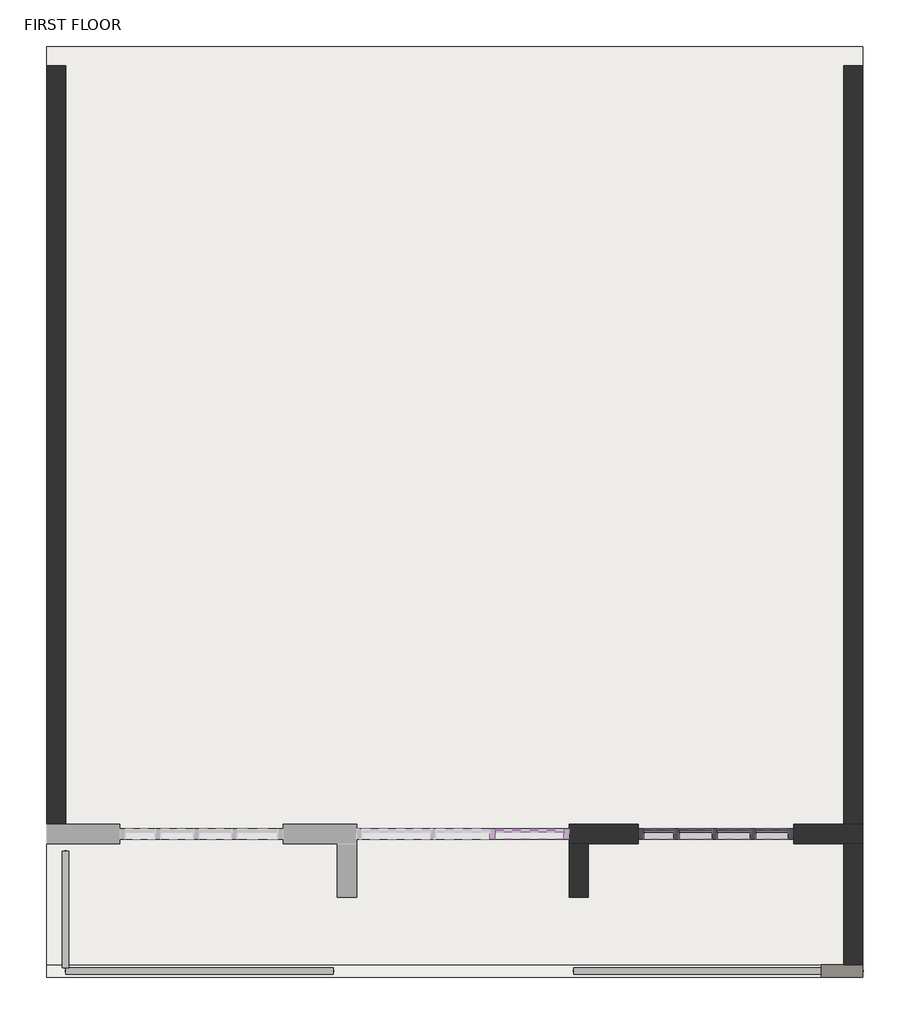
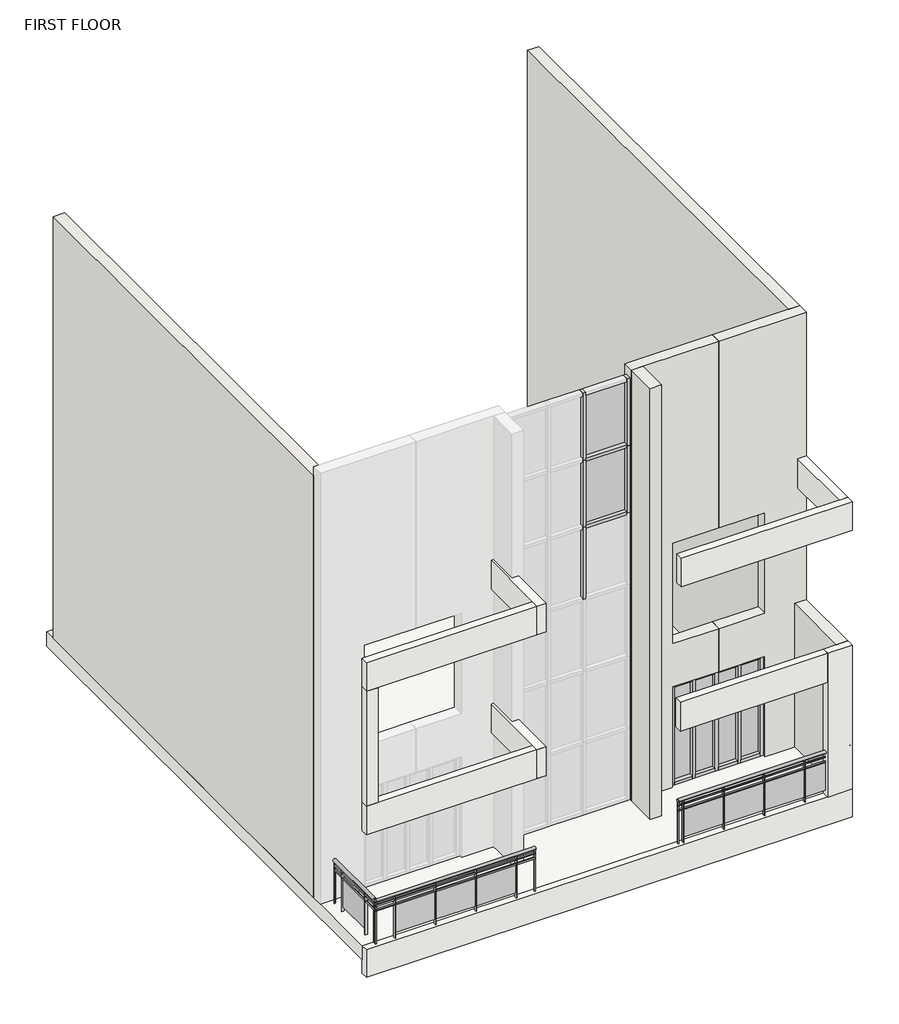
# One storey, part 2 of 2: 33 members, 10 plates, 6 walls, 3 railings, 2 slabs.
"""IFC4 building model written with IfcOpenShell, lengths in millimetres."""

from ifc_helpers import new_model, si_unit, point, frame, origin, place, context, project, spatial, polyline, ellipse_curve, trimmed, outline, extrude, faceted_brep, transform, mapped, element, save
from ifc_brep_helpers import plane_surface, extruded_surface, advanced_brep
from components import member_3374d9b6, member_ad567e07, member_82905deb, member_0514ece2, member_5493b72c, member_7cbddb58, member_843225dc, member_7096a90e, member_75a0f14a, system_panel_glazed_3f785c8f, system_panel_glazed_d91b2d6b, system_panel_glazed_935821d8, system_panel_glazed_f3f5655f, system_panel_glazed_451412b5, floors_1_floors_1_452276dc

model = new_model("IFC4")

# Units and contexts
model_context = context("Model", 3, world=origin())
ifc_project = project(units=[si_unit("LENGTHUNIT", "METRE", prefix="MILLI")], contexts=[model_context])

# Site, building, storey
site = spatial("IfcSite", under=ifc_project)
building = spatial("IfcBuilding", under=site)
storey = spatial("IfcBuildingStorey", under=building, Name="FIRST FLOOR", Elevation=3048.0)

# Members
placement = place(None, origin())
member_shape = member_3374d9b6(model_context)
element("IfcMember", 1, ObjectType="Rectangular Mullion : 2.5\" x 5\" rectangular", at=placement, inside=storey, context=model_context, shape_type="MappedRepresentation", body=[
    mapped(member_shape, transform((2606.0769214, -508.3464931, 3048.0), x_axis=(1.0, 0.0, 0.0), y_axis=(0.0, -1.0, 0.0), z_axis=(0.0, 0.0, -1.0))),
])
element("IfcMember", 2, ObjectType="Rectangular Mullion : 2.5\" x 5\" rectangular", at=placement, inside=storey, context=model_context, shape_type="MappedRepresentation", body=[
    mapped(member_shape, transform((2606.0769214, -508.3464931, 3048.0), x_axis=(1.0, 0.0, 0.0), y_axis=(0.0, -1.0, 0.0), z_axis=(0.0, 0.0, -1.0))),
])
element("IfcMember", 3, ObjectType="Rectangular Mullion : 2.5\" x 5\" rectangular", at=placement, inside=storey, context=model_context, shape_type="MappedRepresentation", body=[
    mapped(member_shape, transform((748.741197, -508.3464931, 5181.6), x_axis=(-1.0, 0.0, 0.0), y_axis=(0.0, -1.0, 0.0), z_axis=(0.0, 0.0, 1.0))),
])
element("IfcMember", 4, ObjectType="Rectangular Mullion : 2.5\" x 5\" rectangular", at=placement, inside=storey, context=model_context, shape_type="MappedRepresentation", body=[
    mapped(member_shape, transform((748.741197, -508.3464931, 5181.6), x_axis=(-1.0, 0.0, 0.0), y_axis=(0.0, -1.0, 0.0), z_axis=(0.0, 0.0, 1.0))),
])
member_2_shape = member_ad567e07(model_context)
element("IfcMember", 5, ObjectType="Rectangular Mullion : 2.5\" x 5\" rectangular", at=placement, inside=storey, context=model_context, shape_type="MappedRepresentation", body=[
    mapped(member_2_shape, transform((-140.258803, -508.3464931, 9144.0), x_axis=(0.0, 0.0, 1.0), y_axis=(0.0, -1.0, 0.0), z_axis=(1.0, 0.0, 0.0))),
])
element("IfcMember", 6, ObjectType="Rectangular Mullion : 2.5\" x 5\" rectangular", at=placement, inside=storey, context=model_context, shape_type="MappedRepresentation", body=[
    mapped(member_2_shape, transform((-140.258803, -508.3464931, 10572.1991558), x_axis=(0.0, 0.0, 1.0), y_axis=(0.0, -1.0, 0.0), z_axis=(1.0, 0.0, 0.0))),
])
member_3_shape = member_82905deb(model_context)
element("IfcMember", 7, ObjectType="Rectangular Mullion : 2.5\" x 5\" rectangular", at=placement, inside=storey, context=model_context, shape_type="MappedRepresentation", body=[
    mapped(member_3_shape, transform((-991.158803, -508.3464931, 7620.0), x_axis=(1.0, 0.0, 0.0), y_axis=(0.0, -1.0, 0.0), z_axis=(0.0, 0.0, -1.0))),
])
member_4_shape = member_0514ece2(model_context)
element("IfcMember", 8, ObjectType="Rectangular Mullion : 2.5\" x 5\" rectangular", at=placement, inside=storey, context=model_context, shape_type="MappedRepresentation", body=[
    mapped(member_4_shape, transform((-991.158803, -508.3464931, 9144.0), x_axis=(1.0, 0.0, 0.0), y_axis=(0.0, -1.0, 0.0), z_axis=(0.0, 0.0, -1.0))),
])
element("IfcMember", 9, ObjectType="Rectangular Mullion : 2.5\" x 5\" rectangular", at=placement, inside=storey, context=model_context, shape_type="MappedRepresentation", body=[
    mapped(member_4_shape, transform((-991.158803, -508.3464931, 10572.1991558), x_axis=(1.0, 0.0, 0.0), y_axis=(0.0, -1.0, 0.0), z_axis=(0.0, 0.0, -1.0))),
])
member_5_shape = member_5493b72c(model_context)
element("IfcMember", 10, ObjectType="Rectangular Mullion : 2.5\" x 5\" rectangular", at=placement, inside=storey, context=model_context, shape_type="MappedRepresentation", body=[
    mapped(member_5_shape, transform((-76.758803, -508.3464931, 9144.0), x_axis=(1.0, 0.0, 0.0), y_axis=(0.0, -1.0, 0.0), z_axis=(0.0, 0.0, -1.0))),
])
element("IfcMember", 11, ObjectType="Rectangular Mullion : 2.5\" x 5\" rectangular", at=placement, inside=storey, context=model_context, shape_type="MappedRepresentation", body=[
    mapped(member_5_shape, transform((-76.758803, -508.3464931, 10572.1991558), x_axis=(1.0, 0.0, 0.0), y_axis=(0.0, -1.0, 0.0), z_axis=(0.0, 0.0, -1.0))),
])
member_6_shape = member_7cbddb58(model_context)
element("IfcMember", 12, ObjectType="Rectangular Mullion : 2.5\" x 5\" rectangular", at=placement, inside=storey, context=model_context, shape_type="MappedRepresentation", body=[
    mapped(member_6_shape, transform((1205.941197, -508.3464931, 3048.0), x_axis=(1.0, 0.0, 0.0), y_axis=(0.0, -1.0, 0.0), z_axis=(0.0, 0.0, -1.0))),
])
element("IfcMember", 13, ObjectType="Rectangular Mullion : 2.5\" x 5\" rectangular", at=placement, inside=storey, context=model_context, shape_type="MappedRepresentation", body=[
    mapped(member_6_shape, transform((1663.141197, -508.3464931, 3048.0), x_axis=(1.0, 0.0, 0.0), y_axis=(0.0, -1.0, 0.0), z_axis=(0.0, 0.0, -1.0))),
])
element("IfcMember", 14, ObjectType="Rectangular Mullion : 2.5\" x 5\" rectangular", at=placement, inside=storey, context=model_context, shape_type="MappedRepresentation", body=[
    mapped(member_6_shape, transform((2120.341197, -508.3464931, 3048.0), x_axis=(1.0, 0.0, 0.0), y_axis=(0.0, -1.0, 0.0), z_axis=(0.0, 0.0, -1.0))),
])
element("IfcMember", 15, ObjectType="Rectangular Mullion : 2.5\" x 5\" rectangular", at=placement, inside=storey, context=model_context, shape_type="MappedRepresentation", body=[
    mapped(member_6_shape, transform((1205.941197, -508.3464931, 3048.0), x_axis=(1.0, 0.0, 0.0), y_axis=(0.0, -1.0, 0.0), z_axis=(0.0, 0.0, -1.0))),
])
element("IfcMember", 16, ObjectType="Rectangular Mullion : 2.5\" x 5\" rectangular", at=placement, inside=storey, context=model_context, shape_type="MappedRepresentation", body=[
    mapped(member_6_shape, transform((1663.141197, -508.3464931, 3048.0), x_axis=(1.0, 0.0, 0.0), y_axis=(0.0, -1.0, 0.0), z_axis=(0.0, 0.0, -1.0))),
])
element("IfcMember", 17, ObjectType="Rectangular Mullion : 2.5\" x 5\" rectangular", at=placement, inside=storey, context=model_context, shape_type="MappedRepresentation", body=[
    mapped(member_6_shape, transform((2120.341197, -508.3464931, 3048.0), x_axis=(1.0, 0.0, 0.0), y_axis=(0.0, -1.0, 0.0), z_axis=(0.0, 0.0, -1.0))),
])
member_7_shape = member_843225dc(model_context)
element("IfcMember", 18, ObjectType="Rectangular Mullion : 2.5\" x 5\" rectangular", at=placement, inside=storey, context=model_context, shape_type="MappedRepresentation", body=[
    mapped(member_7_shape, transform((812.241197, -508.3464931, 3048.0), x_axis=(0.0, 0.0, -1.0), y_axis=(0.0, -1.0, 0.0), z_axis=(-1.0, 0.0, 0.0))),
])
element("IfcMember", 19, ObjectType="Rectangular Mullion : 2.5\" x 5\" rectangular", at=placement, inside=storey, context=model_context, shape_type="MappedRepresentation", body=[
    mapped(member_7_shape, transform((812.241197, -508.3464931, 3048.0), x_axis=(0.0, 0.0, -1.0), y_axis=(0.0, -1.0, 0.0), z_axis=(-1.0, 0.0, 0.0))),
])
element("IfcMember", 20, ObjectType="Rectangular Mullion : 2.5\" x 5\" rectangular", at=placement, inside=storey, context=model_context, shape_type="MappedRepresentation", body=[
    mapped(member_7_shape, transform((1174.191197, -508.3464931, 5181.6), x_axis=(0.0, 0.0, 1.0), y_axis=(0.0, -1.0, 0.0), z_axis=(1.0, 0.0, 0.0))),
])
element("IfcMember", 21, ObjectType="Rectangular Mullion : 2.5\" x 5\" rectangular", at=placement, inside=storey, context=model_context, shape_type="MappedRepresentation", body=[
    mapped(member_7_shape, transform((1174.191197, -508.3464931, 5181.6), x_axis=(0.0, 0.0, 1.0), y_axis=(0.0, -1.0, 0.0), z_axis=(1.0, 0.0, 0.0))),
])
member_8_shape = member_7096a90e(model_context)
element("IfcMember", 22, ObjectType="Rectangular Mullion : 2.5\" x 5\" rectangular", at=placement, inside=storey, context=model_context, shape_type="MappedRepresentation", body=[
    mapped(member_8_shape, transform((1237.691197, -508.3464931, 3048.0), x_axis=(0.0, 0.0, -1.0), y_axis=(0.0, -1.0, 0.0), z_axis=(-1.0, 0.0, 0.0))),
])
element("IfcMember", 23, ObjectType="Rectangular Mullion : 2.5\" x 5\" rectangular", at=placement, inside=storey, context=model_context, shape_type="MappedRepresentation", body=[
    mapped(member_8_shape, transform((1694.891197, -508.3464931, 3048.0), x_axis=(0.0, 0.0, -1.0), y_axis=(0.0, -1.0, 0.0), z_axis=(-1.0, 0.0, 0.0))),
])
element("IfcMember", 24, ObjectType="Rectangular Mullion : 2.5\" x 5\" rectangular", at=placement, inside=storey, context=model_context, shape_type="MappedRepresentation", body=[
    mapped(member_8_shape, transform((1237.691197, -508.3464931, 3048.0), x_axis=(0.0, 0.0, -1.0), y_axis=(0.0, -1.0, 0.0), z_axis=(-1.0, 0.0, 0.0))),
])
element("IfcMember", 25, ObjectType="Rectangular Mullion : 2.5\" x 5\" rectangular", at=placement, inside=storey, context=model_context, shape_type="MappedRepresentation", body=[
    mapped(member_8_shape, transform((1694.891197, -508.3464931, 3048.0), x_axis=(0.0, 0.0, -1.0), y_axis=(0.0, -1.0, 0.0), z_axis=(-1.0, 0.0, 0.0))),
])
element("IfcMember", 26, ObjectType="Rectangular Mullion : 2.5\" x 5\" rectangular", at=placement, inside=storey, context=model_context, shape_type="MappedRepresentation", body=[
    mapped(member_8_shape, transform((1631.391197, -508.3464931, 5181.6), x_axis=(0.0, 0.0, 1.0), y_axis=(0.0, -1.0, 0.0), z_axis=(1.0, 0.0, 0.0))),
])
element("IfcMember", 27, ObjectType="Rectangular Mullion : 2.5\" x 5\" rectangular", at=placement, inside=storey, context=model_context, shape_type="MappedRepresentation", body=[
    mapped(member_8_shape, transform((2088.591197, -508.3464931, 5181.6), x_axis=(0.0, 0.0, 1.0), y_axis=(0.0, -1.0, 0.0), z_axis=(1.0, 0.0, 0.0))),
])
element("IfcMember", 28, ObjectType="Rectangular Mullion : 2.5\" x 5\" rectangular", at=placement, inside=storey, context=model_context, shape_type="MappedRepresentation", body=[
    mapped(member_8_shape, transform((1631.391197, -508.3464931, 5181.6), x_axis=(0.0, 0.0, 1.0), y_axis=(0.0, -1.0, 0.0), z_axis=(1.0, 0.0, 0.0))),
])
element("IfcMember", 29, ObjectType="Rectangular Mullion : 2.5\" x 5\" rectangular", at=placement, inside=storey, context=model_context, shape_type="MappedRepresentation", body=[
    mapped(member_8_shape, transform((2088.591197, -508.3464931, 5181.6), x_axis=(0.0, 0.0, 1.0), y_axis=(0.0, -1.0, 0.0), z_axis=(1.0, 0.0, 0.0))),
])
member_9_shape = member_75a0f14a(model_context)
element("IfcMember", 30, ObjectType="Rectangular Mullion : 2.5\" x 5\" rectangular", at=placement, inside=storey, context=model_context, shape_type="MappedRepresentation", body=[
    mapped(member_9_shape, transform((2542.5769214, -508.3464931, 5181.6), x_axis=(0.0, 0.0, 1.0), y_axis=(0.0, -1.0, 0.0), z_axis=(1.0, 0.0, 0.0))),
])
element("IfcMember", 31, ObjectType="Rectangular Mullion : 2.5\" x 5\" rectangular", at=placement, inside=storey, context=model_context, shape_type="MappedRepresentation", body=[
    mapped(member_9_shape, transform((2542.5769214, -508.3464931, 5181.6), x_axis=(0.0, 0.0, 1.0), y_axis=(0.0, -1.0, 0.0), z_axis=(1.0, 0.0, 0.0))),
])
element("IfcMember", 32, ObjectType="Rectangular Mullion : 2.5\" x 5\" rectangular", at=placement, inside=storey, context=model_context, shape_type="MappedRepresentation", body=[
    mapped(member_9_shape, transform((2152.091197, -508.3464931, 3048.0), x_axis=(0.0, 0.0, -1.0), y_axis=(0.0, -1.0, 0.0), z_axis=(-1.0, 0.0, 0.0))),
])
element("IfcMember", 33, ObjectType="Rectangular Mullion : 2.5\" x 5\" rectangular", at=placement, inside=storey, context=model_context, shape_type="MappedRepresentation", body=[
    mapped(member_9_shape, transform((2152.091197, -508.3464931, 3048.0), x_axis=(0.0, 0.0, -1.0), y_axis=(0.0, -1.0, 0.0), z_axis=(-1.0, 0.0, 0.0))),
])

# Plates
system_panel_glazed_shape = system_panel_glazed_3f785c8f(model_context)
element("IfcPlate", 34, ObjectType="System Panel : Glazed", at=placement, inside=storey, context=model_context, shape_type="MappedRepresentation", body=[
    mapped(system_panel_glazed_shape, transform((-549.833803, -508.3464931, 9175.75), x_axis=(1.0, 0.0, 0.0), y_axis=(0.0, 1.0, 0.0), z_axis=(0.0, 0.0, 1.0))),
])
system_panel_glazed_2_shape = system_panel_glazed_d91b2d6b(model_context)
element("IfcPlate", 35, ObjectType="System Panel : Glazed", at=placement, inside=storey, context=model_context, shape_type="MappedRepresentation", body=[
    mapped(system_panel_glazed_2_shape, transform((-549.833803, -508.3464931, 10603.9491558), x_axis=(1.0, 0.0, 0.0), y_axis=(0.0, 1.0, 0.0), z_axis=(0.0, 0.0, 1.0))),
])
system_panel_glazed_3_shape = system_panel_glazed_935821d8(model_context)
element("IfcPlate", 36, ObjectType="System Panel : Glazed", at=placement, inside=storey, context=model_context, shape_type="MappedRepresentation", body=[
    mapped(system_panel_glazed_3_shape, transform((993.216197, -508.3464931, 3111.5), x_axis=(1.0, 0.0, 0.0), y_axis=(0.0, 1.0, 0.0), z_axis=(0.0, 0.0, 1.0))),
])
element("IfcPlate", 37, ObjectType="System Panel : Glazed", at=placement, inside=storey, context=model_context, shape_type="MappedRepresentation", body=[
    mapped(system_panel_glazed_3_shape, transform((993.216197, -508.3464931, 3111.5), x_axis=(1.0, 0.0, 0.0), y_axis=(0.0, 1.0, 0.0), z_axis=(0.0, 0.0, 1.0))),
])
system_panel_glazed_4_shape = system_panel_glazed_f3f5655f(model_context)
element("IfcPlate", 38, ObjectType="System Panel : Glazed", at=placement, inside=storey, context=model_context, shape_type="MappedRepresentation", body=[
    mapped(system_panel_glazed_4_shape, transform((1434.541197, -508.3464931, 3111.5), x_axis=(1.0, 0.0, 0.0), y_axis=(0.0, 1.0, 0.0), z_axis=(0.0, 0.0, 1.0))),
])
element("IfcPlate", 39, ObjectType="System Panel : Glazed", at=placement, inside=storey, context=model_context, shape_type="MappedRepresentation", body=[
    mapped(system_panel_glazed_4_shape, transform((1891.741197, -508.3464931, 3111.5), x_axis=(1.0, 0.0, 0.0), y_axis=(0.0, 1.0, 0.0), z_axis=(0.0, 0.0, 1.0))),
])
element("IfcPlate", 40, ObjectType="System Panel : Glazed", at=placement, inside=storey, context=model_context, shape_type="MappedRepresentation", body=[
    mapped(system_panel_glazed_4_shape, transform((1434.541197, -508.3464931, 3111.5), x_axis=(1.0, 0.0, 0.0), y_axis=(0.0, 1.0, 0.0), z_axis=(0.0, 0.0, 1.0))),
])
element("IfcPlate", 41, ObjectType="System Panel : Glazed", at=placement, inside=storey, context=model_context, shape_type="MappedRepresentation", body=[
    mapped(system_panel_glazed_4_shape, transform((1891.741197, -508.3464931, 3111.5), x_axis=(1.0, 0.0, 0.0), y_axis=(0.0, 1.0, 0.0), z_axis=(0.0, 0.0, 1.0))),
])
system_panel_glazed_5_shape = system_panel_glazed_451412b5(model_context)
element("IfcPlate", 42, ObjectType="System Panel : Glazed", at=placement, inside=storey, context=model_context, shape_type="MappedRepresentation", body=[
    mapped(system_panel_glazed_5_shape, transform((2347.3340592, -508.3464931, 3111.5), x_axis=(1.0, 0.0, 0.0), y_axis=(0.0, 1.0, 0.0), z_axis=(0.0, 0.0, 1.0))),
])
element("IfcPlate", 43, ObjectType="System Panel : Glazed", at=placement, inside=storey, context=model_context, shape_type="MappedRepresentation", body=[
    mapped(system_panel_glazed_5_shape, transform((2347.3340592, -508.3464931, 3111.5), x_axis=(1.0, 0.0, 0.0), y_axis=(0.0, 1.0, 0.0), z_axis=(0.0, 0.0, 1.0))),
])

# Railings
element("IfcRailing", 44, ObjectType="Glass Panel - Bottom Fill", at=placement, inside=storey, context=model_context, shape_type="SolidModel", body=[
    advanced_brep(
    [(-6093.4230786, -2108.5464178, 3962.4), (-6093.4230786, -2184.7464178, 3962.4), (-2893.0230786, -2108.5464178, 3962.4), (-2893.0230786, -2184.7464178, 3962.4)],
    [
        (0, 1, ellipse_curve(frame((-6093.4230786, -2146.6464178, 3962.4), z_axis=(-1.0, 0.0, 0.0), x_axis=(0.0, -1.0, 0.0)), 38.1, 28.575)),
        (1, 0, ellipse_curve(frame((-6093.4230786, -2146.6464178, 3962.4), z_axis=(-1.0, 0.0, 0.0), x_axis=(0.0, -1.0, 0.0)), 38.1, 28.575)),
        (2, 3, ellipse_curve(frame((-2893.0230786, -2146.6464178, 3962.4), z_axis=(1.0, 0.0, 0.0), x_axis=(0.0, -1.0, 0.0)), 38.1, 28.575)),
        (3, 2, ellipse_curve(frame((-2893.0230786, -2146.6464178, 3962.4), z_axis=(1.0, 0.0, 0.0), x_axis=(0.0, -1.0, 0.0)), 38.1, 28.575)),
        (0, 2),
        (3, 1),
    ],
    [
        plane_surface(frame((-6093.4230786, -2146.6464178, 3962.4), z_axis=(-1.0, 0.0, 0.0), x_axis=(0.0, 1.0, 0.0))),
        plane_surface(frame((-2893.0230786, -2146.6464178, 3962.4), z_axis=(1.0, 0.0, 0.0), x_axis=(0.0, 1.0, 0.0))),
        extruded_surface(trimmed(ellipse_curve(frame((-2893.0230786, -2146.6464178, 3962.4), z_axis=(-1.0, 0.0, 0.0), x_axis=(0.0, -1.0, 0.0)), 38.1, 28.575), [point((-2893.0230786, -2108.5464178, 3962.4))], [point((-2893.0230786, -2184.7464178, 3962.4))], True, "CARTESIAN"), (-3200.3999999999996, 0.0, 0.0), 3200.3999999999996),
        extruded_surface(trimmed(ellipse_curve(frame((-2893.0230786, -2146.6464178, 3962.4), z_axis=(-1.0, 0.0, 0.0), x_axis=(0.0, -1.0, 0.0)), 38.1, 28.575), [point((-2893.0230786, -2184.7464178, 3962.4))], [point((-2893.0230786, -2108.5464178, 3962.4))], True, "CARTESIAN"), (-3200.3999999999996, 0.0, 0.0), 3200.3999999999996),
    ],
    [
        (0, [[1, 2]]),
        (1, [[3, 4]]),
        (2, [[-1, 5, -4, 6]]),
        (3, [[-2, -6, -3, -5]]),
    ],
),
    extrude(outline(polyline([(-6093.4230786, -2159.3464178), (-6093.4230786, -2133.9464178), (-2893.0230786, -2133.9464178), (-2893.0230786, -2159.3464178), (-6093.4230786, -2159.3464178)])), frame((0.0, 0.0, 3848.1), z_axis=(0.0, 0.0, 1.0), x_axis=(1.0, 0.0, 0.0)), (0.0, 0.0, 1.0), 25.4),
    extrude(outline(polyline([(-6093.4230786, -2159.3464178), (-6093.4230786, -2133.9464178), (-2893.0230786, -2133.9464178), (-2893.0230786, -2159.3464178), (-6093.4230786, -2159.3464178)])), frame((0.0, 0.0, 3746.5), z_axis=(0.0, 0.0, 1.0), x_axis=(1.0, 0.0, 0.0)), (0.0, 0.0, 1.0), 25.4),
    extrude(outline(polyline([(-3280.3730786, -2172.0464178), (-3280.3730786, -2121.2464178), (-3267.6730786, -2121.2464178), (-3267.6730786, -2172.0464178), (-3280.3730786, -2172.0464178)])), frame((0.0, 0.0, 3048.0), z_axis=(0.0, 0.0, 1.0), x_axis=(1.0, 0.0, 0.0)), (0.0, 0.0, 1.0), 885.6788223),
    extrude(outline(polyline([(-4086.8230786, -2140.1112608), (-3274.0230786, -2140.1112608), (-3274.0230786, -2146.4612608), (-4086.8230786, -2146.4612608), (-4086.8230786, -2140.1112608)])), frame((0.0, 0.0, 3149.6), z_axis=(0.0, 0.0, 1.0), x_axis=(1.0, 0.0, 0.0)), (0.0, 0.0, 1.0), 596.9),
    extrude(outline(polyline([(-4093.1730786, -2172.0464178), (-4093.1730786, -2121.2464178), (-4080.4730786, -2121.2464178), (-4080.4730786, -2172.0464178), (-4093.1730786, -2172.0464178)])), frame((0.0, 0.0, 3048.0), z_axis=(0.0, 0.0, 1.0), x_axis=(1.0, 0.0, 0.0)), (0.0, 0.0, 1.0), 885.6788223),
    extrude(outline(polyline([(-4899.6230786, -2140.1112608), (-4086.8230786, -2140.1112608), (-4086.8230786, -2146.4612608), (-4899.6230786, -2146.4612608), (-4899.6230786, -2140.1112608)])), frame((0.0, 0.0, 3149.6), z_axis=(0.0, 0.0, 1.0), x_axis=(1.0, 0.0, 0.0)), (0.0, 0.0, 1.0), 596.9),
    extrude(outline(polyline([(-4905.9730786, -2172.0464178), (-4905.9730786, -2121.2464178), (-4893.2730786, -2121.2464178), (-4893.2730786, -2172.0464178), (-4905.9730786, -2172.0464178)])), frame((0.0, 0.0, 3048.0), z_axis=(0.0, 0.0, 1.0), x_axis=(1.0, 0.0, 0.0)), (0.0, 0.0, 1.0), 885.6788223),
    extrude(outline(polyline([(-5712.4230786, -2140.1112608), (-4899.6230786, -2140.1112608), (-4899.6230786, -2146.4612608), (-5712.4230786, -2146.4612608), (-5712.4230786, -2140.1112608)])), frame((0.0, 0.0, 3149.6), z_axis=(0.0, 0.0, 1.0), x_axis=(1.0, 0.0, 0.0)), (0.0, 0.0, 1.0), 596.9),
    extrude(outline(polyline([(-5718.7730786, -2172.0464178), (-5718.7730786, -2121.2464178), (-5706.0730786, -2121.2464178), (-5706.0730786, -2172.0464178), (-5718.7730786, -2172.0464178)])), frame((0.0, 0.0, 3048.0), z_axis=(0.0, 0.0, 1.0), x_axis=(1.0, 0.0, 0.0)), (0.0, 0.0, 1.0), 885.6788223),
    extrude(outline(polyline([(-2905.7230786, -2156.1714178), (-2905.7230786, -2137.1214178), (-2886.6730786, -2137.1214178), (-2886.6730786, -2156.1714178), (-2905.7230786, -2156.1714178)])), frame((0.0, 0.0, 3048.0), z_axis=(0.0, 0.0, 1.0), x_axis=(1.0, 0.0, 0.0)), (0.0, 0.0, 1.0), 885.6788223),
    extrude(outline(polyline([(-6099.7730786, -2156.1714178), (-6099.7730786, -2137.1214178), (-6080.7230786, -2137.1214178), (-6080.7230786, -2156.1714178), (-6099.7730786, -2156.1714178)])), frame((0.0, 0.0, 3048.0), z_axis=(0.0, 0.0, 1.0), x_axis=(1.0, 0.0, 0.0)), (0.0, 0.0, 1.0), 885.6788223),
])
element("IfcRailing", 45, ObjectType="Glass Panel - Bottom Fill", at=placement, inside=storey, context=model_context, shape_type="SolidModel", body=[
    advanced_brep(
    [(-22.6504261, -2108.5464178, 3962.4), (-22.6504261, -2184.7464178, 3962.4), (3431.5769214, -2108.5464178, 3962.4), (3431.5769214, -2184.7464178, 3962.4)],
    [
        (0, 1, ellipse_curve(frame((-22.6504261, -2146.6464178, 3962.4), z_axis=(-1.0, 0.0, 0.0), x_axis=(0.0, -1.0, 0.0)), 38.1, 28.575)),
        (1, 0, ellipse_curve(frame((-22.6504261, -2146.6464178, 3962.4), z_axis=(-1.0, 0.0, 0.0), x_axis=(0.0, -1.0, 0.0)), 38.1, 28.575)),
        (2, 3, ellipse_curve(frame((3431.5769214, -2146.6464178, 3962.4), z_axis=(1.0, 0.0, 0.0), x_axis=(0.0, -1.0, 0.0)), 38.1, 28.575)),
        (3, 2, ellipse_curve(frame((3431.5769214, -2146.6464178, 3962.4), z_axis=(1.0, 0.0, 0.0), x_axis=(0.0, -1.0, 0.0)), 38.1, 28.575)),
        (0, 2),
        (3, 1),
    ],
    [
        plane_surface(frame((-22.6504261, -2146.6464178, 3962.4), z_axis=(-1.0, 0.0, 0.0), x_axis=(0.0, 1.0, 0.0))),
        plane_surface(frame((3431.5769214, -2146.6464178, 3962.4), z_axis=(1.0, 0.0, 0.0), x_axis=(0.0, 1.0, 0.0))),
        extruded_surface(trimmed(ellipse_curve(frame((3431.5769214, -2146.6464178, 3962.4), z_axis=(-1.0, 0.0, 0.0), x_axis=(0.0, -1.0, 0.0)), 38.1, 28.575), [point((3431.5769214, -2108.5464178, 3962.4))], [point((3431.5769214, -2184.7464178, 3962.4))], True, "CARTESIAN"), (-3454.2273475, 0.0, 0.0), 3454.2273475),
        extruded_surface(trimmed(ellipse_curve(frame((3431.5769214, -2146.6464178, 3962.4), z_axis=(-1.0, 0.0, 0.0), x_axis=(0.0, -1.0, 0.0)), 38.1, 28.575), [point((3431.5769214, -2184.7464178, 3962.4))], [point((3431.5769214, -2108.5464178, 3962.4))], True, "CARTESIAN"), (-3454.2273475, 0.0, 0.0), 3454.2273475),
    ],
    [
        (0, [[1, 2]]),
        (1, [[3, 4]]),
        (2, [[-1, 5, -4, 6]]),
        (3, [[-2, -6, -3, -5]]),
    ],
),
    extrude(outline(polyline([(-22.6504261, -2159.3464178), (-22.6504261, -2133.9464178), (3431.5769214, -2133.9464178), (3431.5769214, -2159.3464178), (-22.6504261, -2159.3464178)])), frame((0.0, 0.0, 3848.1), z_axis=(0.0, 0.0, 1.0), x_axis=(1.0, 0.0, 0.0)), (0.0, 0.0, 1.0), 25.4),
    extrude(outline(polyline([(-22.6504261, -2159.3464178), (-22.6504261, -2133.9464178), (3431.5769214, -2133.9464178), (3431.5769214, -2159.3464178), (-22.6504261, -2159.3464178)])), frame((0.0, 0.0, 3746.5), z_axis=(0.0, 0.0, 1.0), x_axis=(1.0, 0.0, 0.0)), (0.0, 0.0, 1.0), 25.4),
    extrude(outline(polyline([(3323.7132477, -2172.0464178), (3323.7132477, -2121.2464178), (3336.4132477, -2121.2464178), (3336.4132477, -2172.0464178), (3323.7132477, -2172.0464178)])), frame((0.0, 0.0, 3048.0), z_axis=(0.0, 0.0, 1.0), x_axis=(1.0, 0.0, 0.0)), (0.0, 0.0, 1.0), 885.6788223),
    extrude(outline(polyline([(2517.2632477, -2140.1112608), (3330.0632477, -2140.1112608), (3330.0632477, -2146.4612608), (2517.2632477, -2146.4612608), (2517.2632477, -2140.1112608)])), frame((0.0, 0.0, 3149.6), z_axis=(0.0, 0.0, 1.0), x_axis=(1.0, 0.0, 0.0)), (0.0, 0.0, 1.0), 596.9),
    extrude(outline(polyline([(2510.9132477, -2172.0464178), (2510.9132477, -2121.2464178), (2523.6132477, -2121.2464178), (2523.6132477, -2172.0464178), (2510.9132477, -2172.0464178)])), frame((0.0, 0.0, 3048.0), z_axis=(0.0, 0.0, 1.0), x_axis=(1.0, 0.0, 0.0)), (0.0, 0.0, 1.0), 885.6788223),
    extrude(outline(polyline([(1704.4632477, -2140.1112608), (2517.2632477, -2140.1112608), (2517.2632477, -2146.4612608), (1704.4632477, -2146.4612608), (1704.4632477, -2140.1112608)])), frame((0.0, 0.0, 3149.6), z_axis=(0.0, 0.0, 1.0), x_axis=(1.0, 0.0, 0.0)), (0.0, 0.0, 1.0), 596.9),
    extrude(outline(polyline([(1698.1132477, -2172.0464178), (1698.1132477, -2121.2464178), (1710.8132477, -2121.2464178), (1710.8132477, -2172.0464178), (1698.1132477, -2172.0464178)])), frame((0.0, 0.0, 3048.0), z_axis=(0.0, 0.0, 1.0), x_axis=(1.0, 0.0, 0.0)), (0.0, 0.0, 1.0), 885.6788223),
    extrude(outline(polyline([(891.6632477, -2140.1112608), (1704.4632477, -2140.1112608), (1704.4632477, -2146.4612608), (891.6632477, -2146.4612608), (891.6632477, -2140.1112608)])), frame((0.0, 0.0, 3149.6), z_axis=(0.0, 0.0, 1.0), x_axis=(1.0, 0.0, 0.0)), (0.0, 0.0, 1.0), 596.9),
    extrude(outline(polyline([(885.3132477, -2172.0464178), (885.3132477, -2121.2464178), (898.0132477, -2121.2464178), (898.0132477, -2172.0464178), (885.3132477, -2172.0464178)])), frame((0.0, 0.0, 3048.0), z_axis=(0.0, 0.0, 1.0), x_axis=(1.0, 0.0, 0.0)), (0.0, 0.0, 1.0), 885.6788223),
    extrude(outline(polyline([(78.8632477, -2140.1112608), (891.6632477, -2140.1112608), (891.6632477, -2146.4612608), (78.8632477, -2146.4612608), (78.8632477, -2140.1112608)])), frame((0.0, 0.0, 3149.6), z_axis=(0.0, 0.0, 1.0), x_axis=(1.0, 0.0, 0.0)), (0.0, 0.0, 1.0), 596.9),
    extrude(outline(polyline([(72.5132477, -2172.0464178), (72.5132477, -2121.2464178), (85.2132477, -2121.2464178), (85.2132477, -2172.0464178), (72.5132477, -2172.0464178)])), frame((0.0, 0.0, 3048.0), z_axis=(0.0, 0.0, 1.0), x_axis=(1.0, 0.0, 0.0)), (0.0, 0.0, 1.0), 885.6788223),
    extrude(outline(polyline([(3418.8769214, -2156.1714178), (3418.8769214, -2137.1214178), (3437.9269214, -2137.1214178), (3437.9269214, -2156.1714178), (3418.8769214, -2156.1714178)])), frame((0.0, 0.0, 3048.0), z_axis=(0.0, 0.0, 1.0), x_axis=(1.0, 0.0, 0.0)), (0.0, 0.0, 1.0), 885.6788223),
    extrude(outline(polyline([(-29.0004261, -2156.1714178), (-29.0004261, -2137.1214178), (-9.9504261, -2137.1214178), (-9.9504261, -2156.1714178), (-29.0004261, -2156.1714178)])), frame((0.0, 0.0, 3048.0), z_axis=(0.0, 0.0, 1.0), x_axis=(1.0, 0.0, 0.0)), (0.0, 0.0, 1.0), 885.6788223),
])
element("IfcRailing", 46, ObjectType="Glass Panel - Bottom Fill", at=placement, inside=storey, context=model_context, shape_type="SolidModel", body=[
    advanced_brep(
    [(-6055.3230786, -716.4841083, 3962.4), (-6131.5230786, -716.4841083, 3962.4), (-6055.3230786, -2107.9661217, 3962.4), (-6131.5230786, -2107.9661217, 3962.4)],
    [
        (0, 1, ellipse_curve(frame((-6093.4230786, -716.4841083, 3962.4), z_axis=(0.0, 1.0, 0.0), x_axis=(-1.0, 0.0, 0.0)), 38.1, 28.575)),
        (1, 0, ellipse_curve(frame((-6093.4230786, -716.4841083, 3962.4), z_axis=(0.0, 1.0, 0.0), x_axis=(-1.0, 0.0, 0.0)), 38.1, 28.575)),
        (2, 3, ellipse_curve(frame((-6093.4230786, -2107.9661217, 3962.4), z_axis=(0.0, -1.0, 0.0), x_axis=(-1.0, 0.0, 0.0)), 38.1, 28.575)),
        (3, 2, ellipse_curve(frame((-6093.4230786, -2107.9661217, 3962.4), z_axis=(0.0, -1.0, 0.0), x_axis=(-1.0, 0.0, 0.0)), 38.1, 28.575)),
        (0, 2),
        (3, 1),
    ],
    [
        plane_surface(frame((-6093.4230786, -716.4841083, 3962.4), z_axis=(0.0, 1.0, 0.0), x_axis=(0.0, 0.0, -1.0))),
        plane_surface(frame((-6093.4230786, -2107.9661217, 3962.4), z_axis=(0.0, -1.0, 0.0), x_axis=(0.0, 0.0, -1.0))),
        extruded_surface(trimmed(ellipse_curve(frame((-6093.4230786, -2107.9661217, 3962.4), z_axis=(0.0, 1.0, 0.0), x_axis=(-1.0, 0.0, 0.0)), 38.1, 28.575), [point((-6055.3230786, -2107.9661217, 3962.4))], [point((-6131.5230786, -2107.9661217, 3962.4))], True, "CARTESIAN"), (0.0, 1391.4820133999997, 0.0), 1391.4820133999997),
        extruded_surface(trimmed(ellipse_curve(frame((-6093.4230786, -2107.9661217, 3962.4), z_axis=(0.0, 1.0, 0.0), x_axis=(-1.0, 0.0, 0.0)), 38.1, 28.575), [point((-6131.5230786, -2107.9661217, 3962.4))], [point((-6055.3230786, -2107.9661217, 3962.4))], True, "CARTESIAN"), (0.0, 1391.4820133999997, 0.0), 1391.4820133999997),
    ],
    [
        (0, [[1, 2]]),
        (1, [[3, 4]]),
        (2, [[-1, 5, -4, 6]]),
        (3, [[-2, -6, -3, -5]]),
    ],
),
    extrude(outline(polyline([(-6106.1230786, -716.4841083), (-6080.7230786, -716.4841083), (-6080.7230786, -2107.9661217), (-6106.1230786, -2107.9661217), (-6106.1230786, -716.4841083)])), frame((0.0, 0.0, 3848.1), z_axis=(0.0, 0.0, 1.0), x_axis=(1.0, 0.0, 0.0)), (0.0, 0.0, 1.0), 25.4),
    extrude(outline(polyline([(-6106.1230786, -716.4841083), (-6080.7230786, -716.4841083), (-6080.7230786, -2107.9661217), (-6106.1230786, -2107.9661217), (-6106.1230786, -716.4841083)])), frame((0.0, 0.0, 3746.5), z_axis=(0.0, 0.0, 1.0), x_axis=(1.0, 0.0, 0.0)), (0.0, 0.0, 1.0), 25.4),
    extrude(outline(polyline([(-6118.8230786, -1812.275115), (-6068.0230786, -1812.275115), (-6068.0230786, -1824.975115), (-6118.8230786, -1824.975115), (-6118.8230786, -1812.275115)])), frame((0.0, 0.0, 3048.0), z_axis=(0.0, 0.0, 1.0), x_axis=(1.0, 0.0, 0.0)), (0.0, 0.0, 1.0), 885.6788223),
    extrude(outline(polyline([(-6086.8879216, -1005.825115), (-6086.8879216, -1818.625115), (-6093.2379216, -1818.625115), (-6093.2379216, -1005.825115), (-6086.8879216, -1005.825115)])), frame((0.0, 0.0, 3149.6), z_axis=(0.0, 0.0, 1.0), x_axis=(1.0, 0.0, 0.0)), (0.0, 0.0, 1.0), 596.9),
    extrude(outline(polyline([(-6118.8230786, -999.475115), (-6068.0230786, -999.475115), (-6068.0230786, -1012.175115), (-6118.8230786, -1012.175115), (-6118.8230786, -999.475115)])), frame((0.0, 0.0, 3048.0), z_axis=(0.0, 0.0, 1.0), x_axis=(1.0, 0.0, 0.0)), (0.0, 0.0, 1.0), 885.6788223),
    extrude(outline(polyline([(-6102.9480786, -2095.2661217), (-6083.8980786, -2095.2661217), (-6083.8980786, -2114.3161217), (-6102.9480786, -2114.3161217), (-6102.9480786, -2095.2661217)])), frame((0.0, 0.0, 3048.0), z_axis=(0.0, 0.0, 1.0), x_axis=(1.0, 0.0, 0.0)), (0.0, 0.0, 1.0), 885.6788223),
    extrude(outline(polyline([(-6102.9480786, -710.1341083), (-6083.8980786, -710.1341083), (-6083.8980786, -729.1841083), (-6102.9480786, -729.1841083), (-6102.9480786, -710.1341083)])), frame((0.0, 0.0, 3048.0), z_axis=(0.0, 0.0, 1.0), x_axis=(1.0, 0.0, 0.0)), (0.0, 0.0, 1.0), 885.6788223),
])

# Slabs
floors_1_floors_1_shape = floors_1_floors_1_452276dc(model_context)
element("IfcSlab", 47, ObjectType="Floors 1 : Floors 1", at=placement, inside=storey, context=model_context, shape_type="MappedRepresentation", body=[
    mapped(floors_1_floors_1_shape, transform((0.0, 0.0, 0.0), x_axis=(1.0, 0.0, 0.0), y_axis=(0.0, 1.0, 0.0), z_axis=(0.0, 0.0, 1.0))),
])
element("IfcSlab", 48, ObjectType="Generic - 12\"", at=placement, inside=storey, context=model_context, shape_type="SweptSolid", body=[
    extrude(outline(polyline([(3431.5769214, -2070.4464178), (-6322.0230786, -2070.4464178), (-6322.0230786, 8902.3535822), (3431.5769214, 8902.3535822), (3431.5769214, -2070.4464178)])), frame((0.0, 0.0, 2743.2), z_axis=(0.0, 0.0, 1.0), x_axis=(1.0, 0.0, 0.0)), (0.0, 0.0, 1.0), 304.8),
])

# Walls
element("IfcWall", 49, ObjectType="9\"", at=placement, inside=storey, context=model_context, shape_type="SweptSolid", body=[
    extrude(outline(polyline([(-6322.0230786, -394.0464931), (-6322.0230786, 8673.7535822), (-6093.4230786, 8673.7535822), (-6093.4230786, -394.0464931), (-6322.0230786, -394.0464931)])), frame((0.0, 0.0, 3048.0), z_axis=(0.0, 0.0, 1.0), x_axis=(1.0, 0.0, 0.0)), (0.0, 0.0, 1.0), 8952.3983116),
])
element("IfcWall", 50, ObjectType="9\"", at=placement, inside=storey, context=model_context, shape_type="SweptSolid", body=[
    extrude(outline(polyline([(3202.9769214, -394.0464931), (3202.9769214, 8673.7535822), (3431.5769214, 8673.7535822), (3431.5769214, -394.0464931), (3202.9769214, -394.0464931)])), frame((0.0, 0.0, 3048.0), z_axis=(0.0, 0.0, 1.0), x_axis=(1.0, 0.0, 0.0)), (0.0, 0.0, 1.0), 9144.0),
])
element("IfcWall", 51, ObjectType="9\"", at=placement, inside=storey, context=model_context, shape_type="SweptSolid", body=[
    extrude(outline(polyline([(3202.9769214, -2070.4464178), (3202.9769214, -622.6464931), (3431.5769214, -622.6464931), (3431.5769214, -2070.4464178), (3202.9769214, -2070.4464178)])), frame((0.0, 0.0, 3048.0), z_axis=(0.0, 0.0, 1.0), x_axis=(1.0, 0.0, 0.0)), (0.0, 0.0, 1.0), 3048.0),
])
element("IfcWall", 52, ObjectType="9\"", at=placement, inside=storey, context=model_context, shape_type="SweptSolid", body=[
    extrude(outline(polyline([(151.841197, -622.6464931), (151.841197, -1267.5217987), (-76.758803, -1267.5217987), (-76.758803, -622.6464931), (151.841197, -622.6464931)])), frame((0.0, 0.0, 3048.0), z_axis=(0.0, 0.0, 1.0), x_axis=(1.0, 0.0, 0.0)), (0.0, 0.0, 1.0), 9144.0),
])
element("IfcWall", 53, ObjectType="9\"", at=placement, inside=storey, context=model_context, shape_type="Brep", body=[
    faceted_brep([(1677.4090592, -622.6464931, 12192.0), (151.841197, -622.6464931, 12192.0), (-76.758803, -622.6464931, 12192.0), (-76.758803, -622.6464931, 3048.0), (151.841197, -622.6464931, 3048.0), (748.741197, -622.6464931, 3048.0), (748.741197, -622.6464931, 5181.6), (1677.4090592, -622.6464931, 5181.6), (1677.4090592, -622.6464931, 6096.0), (748.741197, -622.6464931, 6096.0), (748.741197, -622.6464931, 8229.6), (1677.4090592, -622.6464931, 8229.6), (-76.758803, -394.0464931, 12192.0), (1677.4090592, -394.0464931, 12192.0), (1677.4090592, -394.0464931, 8229.6), (748.741197, -394.0464931, 8229.6), (748.741197, -394.0464931, 6096.0), (1677.4090592, -394.0464931, 6096.0), (1677.4090592, -394.0464931, 5181.6), (748.741197, -394.0464931, 5181.6), (748.741197, -394.0464931, 3048.0), (-76.758803, -394.0464931, 3048.0)], [[[0, 1, 2, 3, 4, 5, 6, 7, 8, 9, 10, 11]], [[12, 13, 14, 15, 16, 17, 18, 19, 20, 21]], [[13, 0, 11, 14]], [[7, 18, 17, 8]], [[2, 1, 0, 13, 12]], [[3, 21, 20, 5, 4]], [[3, 2, 12, 21]], [[19, 6, 5, 20]], [[6, 19, 18, 7]], [[9, 16, 15, 10]], [[10, 15, 14, 11]], [[16, 9, 8, 17]]]),
])
element("IfcWall", 54, ObjectType="9\"", at=placement, inside=storey, context=model_context, shape_type="Brep", body=[
    faceted_brep([(3431.5769214, -622.6464931, 12192.0), (1677.4090592, -622.6464931, 12192.0), (1677.4090592, -622.6464931, 8229.6), (2606.0769214, -622.6464931, 8229.6), (2606.0769214, -622.6464931, 6096.0), (1677.4090592, -622.6464931, 6096.0), (1677.4090592, -622.6464931, 5181.6), (2606.0769214, -622.6464931, 5181.6), (2606.0769214, -622.6464931, 3048.0), (3202.9769214, -622.6464931, 3048.0), (3431.5769214, -622.6464931, 3048.0), (3431.5769214, -622.6464931, 6096.0), (1677.4090592, -394.0464931, 12192.0), (3202.9769214, -394.0464931, 12192.0), (3431.5769214, -394.0464931, 12192.0), (3431.5769214, -394.0464931, 3048.0), (3202.9769214, -394.0464931, 3048.0), (2606.0769214, -394.0464931, 3048.0), (2606.0769214, -394.0464931, 5181.6), (1677.4090592, -394.0464931, 5181.6), (1677.4090592, -394.0464931, 6096.0), (2606.0769214, -394.0464931, 6096.0), (2606.0769214, -394.0464931, 8229.6), (1677.4090592, -394.0464931, 8229.6)], [[[0, 1, 2, 3, 4, 5, 6, 7, 8, 9, 10, 11]], [[12, 13, 14, 15, 16, 17, 18, 19, 20, 21, 22, 23]], [[1, 0, 14, 13, 12]], [[15, 10, 9, 8, 17, 16]], [[1, 12, 23, 2]], [[19, 6, 5, 20]], [[10, 15, 14, 0, 11]], [[18, 7, 6, 19]], [[7, 18, 17, 8]], [[22, 3, 2, 23]], [[3, 22, 21, 4]], [[4, 21, 20, 5]]]),
])

save(model, "model.ifc")

# Revit data of these elements
# Type "Rectangular Mullion : 2.5\" x 5\" rectangular"
#   built-in parameter 1007304 = 0.416667 (stored number, unit not read)
#   built-in parameter 1007301 = 0.104167 (stored number, unit not read)
#   built-in parameter 1007300 = 0.104167 (stored number, unit not read)
# Type "System Panel : Glazed"
#   Construction Type Id = "GSP4R"
#   Analytic Construction = "1/8 in Pilkington single glazing"
#   Visual Light Transmittance = 0.9
#   Solar Heat Gain Coefficient = 0.86
#   Heat Transfer Coefficient (U) = 1.18115 BTU/(h·ft²·°F)
#   Define Thermal Properties by = 1
# Type "Glass Panel - Bottom Fill"
#   Assembly Code = "C2010400"
#   built-in parameter 1008612 = 0.0416667 (stored number, unit not read)
#   built-in parameter 1008611 = 0.0416667 (stored number, unit not read)
#   built-in parameter 1008609 = 0.333333 (stored number, unit not read)
#   built-in parameter 1008604 = 0.166667 (stored number, unit not read)
#   built-in parameter 1008603 = 0.166667 (stored number, unit not read)
#   Railing Height = 3' - 0"
#   built-in parameter 1008630 = 2
#   built-in parameter 1008610 = 2
#   built-in parameter 1008618 = Baluster - Square : 3/4"
# Type "Generic - 12\""
#   Assembly Code = "B1010"
#   Function = 0
#   Layers, outside or top first: 1' - 0" no material (function 1)
# Type "9\""
#   Assembly Code = "B2010"
#   Layers, outside or top first: 0' - 9" no material (function 1)
# Elements 1, 2, 3, 4, 5, 6, 7, 8, 9, 10, 11, 12, 13, 14, 15, 16, 17, 18, 19, 20, 21, 22, 23, 24, 25, 26, 27, 28, 29, 30, 31, 32, 33 (IfcMember, "Rectangular Mullion : 2.5\" x 5\" rectangular")
#   Phase Created = New Construction
#   Materials on its faces: "Aluminum"
# Elements 34, 35, 36, 37, 38, 39, 40, 41, 42, 43 (IfcPlate, "System Panel : Glazed")
#   Phase Created = New Construction
#   Materials on its faces: "Glass"
# Elements 44, 45, 46 (IfcRailing, "Glass Panel - Bottom Fill")
#   Phase Created = New Construction
#   Materials on its faces: "Glass"
# Element 47 (IfcSlab, "Floors 1 : Floors 1")
#   Phase Created = New Construction
#   Materials on its faces: "Default Floor", "1 wall"
# Element 48 (IfcSlab, "Generic - 12\"")
#   Height Offset From Level = 0' - 0"
#   Phase Created = New Construction
#   Materials on its faces: "Default Floor"
# Elements 49, 50, 53, 54 (IfcWall, "9\"")
#   Top Offset = 0' - 0"
#   Base Offset = 0' - 0"
#   wall height = 30' - 0"
#   Phase Created = New Construction
#   Base Constraint = FIRST FLOOR
#   Top Constraint = FOURTH FLOOR
#   Materials on its faces: "Default Wall", "1 wall"
# Element 51 (IfcWall, "9\"")
#   Top Offset = 0' - 0"
#   Base Offset = 0' - 0"
#   Unconnected Height = 10' - 0"
#   wall height = 10' - 0"
#   Phase Created = New Construction
#   Base Constraint = FIRST FLOOR
#   Materials on its faces: "Default Wall", "1 wall"
# Element 52 (IfcWall, "9\"")
#   Top Offset = 0' - 0"
#   Base Offset = 0' - 0"
#   wall height = 30' - 0"
#   Phase Created = New Construction
#   Base Constraint = FIRST FLOOR
#   Top Constraint = FOURTH FLOOR
#   Materials on its faces: "Default Wall"
# Materials
#   "Aluminum": class "Metal", colour RGB 247 247 247, transparency 0, Description = "Aluminum 6061", Cost = 0
#   "Glass": class "Glass", colour RGB 0 128 192, transparency 0.75, Description = "Soda Lime Glass", Cost = 0
#   "Default Floor": colour RGB 128 128 128, transparency 0, Cost = 0
#   "1 wall": class "Generic", colour RGB 244 245 241, transparency 0, Cost = 0
#   "Default Wall": colour RGB 128 128 128, transparency 0, Cost = 0
